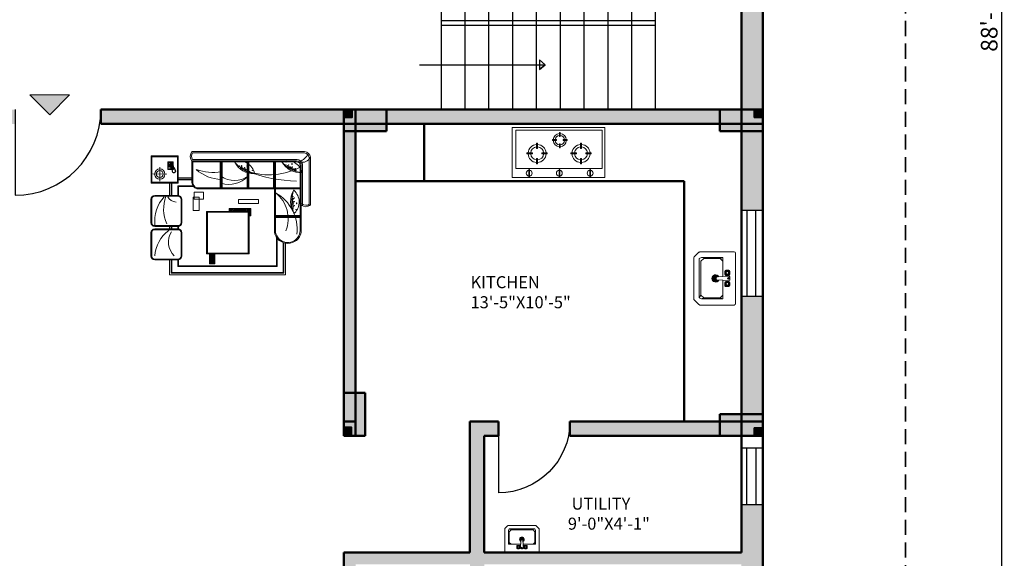
# Model space of a CAD drawing. Units: inches. Extents: x -7 to 1228, y -146 to 1091.
# Tile 42 of 88: x 815 to 1228, y 304 to 531. Entities that reach past the tile are written whole.
import ezdxf

# ---------------------------------------------------------------- set-up
doc = ezdxf.new("R2010")
doc.units = ezdxf.units.IN
doc.linetypes.add('DASHED2', pattern=[9.525, 6.35, -3.175])
for name, color, linetype, lineweight in [('A-ANNO-DIMS', 2, 'Continuous', 18), ('A-ANNO-SYMB', 30, 'Continuous', 18), ('A-AREA-IDEN', 7, 'Continuous', 18), ('A-COLS', 6, 'Continuous', 35), ('A-DOOR', 4, 'Continuous', 25), ('A-FLOR-STRS', 1, 'Continuous', 25), ('A-FURN', 8, 'Continuous', 18), ('A-GLAZ', 175, 'Continuous', 25), ('A-WALL', 7, 'Continuous', 50), ('A-WALL-PATT', 251, 'Continuous', 13), ('C-PROP', 1, 'DASHED2', 35)]:
    doc.layers.add(name, color=color, linetype=linetype, lineweight=lineweight)
doc.styles.get("Standard").update_dxf_attribs({"font": 'arial.ttf'})
doc.dimstyles.new('ISO-25', dxfattribs={"dimtxt": 7, "dimasz": 4, "dimexe": 1.25, "dimexo": 0.625, "dimtad": 1, "dimdec": 1, "dimlunit": 3, "dimtxsty": 'Standard', "dimcen": 2.5, "dimadec": 0, "dimazin": 0, "dimtfac": 1, "dimtdec": 1, "dimtmove": 1, "dimatfit": 3, "dimfxl": 1, "dimarcsym": 0})

# ---------------------------------------------------------------- blocks, each defined once
blk = doc.blocks.new('A$C72243D80')
at = {"ltscale": 1000}
for p, q in [((0, 0), (0, 384.2)), ((0, 384.2), (712, 384.2)), ((712, 384.2), (712, 0)), ((29.5, 68.9), (29.5, 363.2)), ((29.5, 363.2), (692.7, 363.2)), ((363.5, 314.5), (363.5, 345.1)), ((363.5, 345.1), (369.5, 345.1)), ((369.5, 314.5), (363.5, 314.5)), ((369.5, 345.1), (369.5, 314.5)), ((692.7, 363.2), (692.7, 68.9)), ((188.1, 264.2), (188.1, 222.1)), ((196.4, 264.2), (188.1, 264.2)), ((196.4, 222.1), (196.4, 264.2)), ((309.4, 291), (340, 291)), ((309.4, 285), (309.4, 291)), ((340, 285), (309.4, 285)), ((340, 291), (340, 285)), ((363.5, 260), (363.5, 229.4)), ((369.5, 260), (363.5, 260)), ((363.5, 229.4), (369.5, 229.4)), ((369.5, 229.4), (369.5, 260)), ((392.3, 291), (392.3, 285)), ((422.9, 291), (392.3, 291)), ((392.3, 285), (422.9, 285)), ((422.9, 285), (422.9, 291)), ((525.9, 222.1), (525.9, 264.2)), ((525.9, 264.2), (534.1, 264.2)), ((534.1, 264.2), (534.1, 222.1)), ((114.7, 189.8), (156.8, 189.8)), ((114.7, 181.6), (114.7, 189.8)), ((156.8, 181.6), (114.7, 181.6)), ((156.8, 189.8), (156.8, 181.6)), ((188.1, 222.1), (196.4, 222.1)), ((228.6, 189.8), (228.6, 181.6)), ((270.7, 189.8), (228.6, 189.8)), ((228.6, 181.6), (270.7, 181.6)), ((270.7, 181.6), (270.7, 189.8)), ((451.5, 189.8), (493.6, 189.8)), ((451.5, 181.6), (451.5, 189.8)), ((493.6, 181.6), (451.5, 181.6)), ((493.6, 189.8), (493.6, 181.6)), ((534.1, 222.1), (525.9, 222.1)), ((565.5, 189.8), (565.5, 181.6)), ((607.6, 189.8), (565.5, 189.8)), ((565.5, 181.6), (607.6, 181.6)), ((607.6, 181.6), (607.6, 189.8)), ((188.1, 147.2), (196.4, 147.2)), ((188.1, 105.1), (188.1, 147.2)), ((196.4, 105.1), (188.1, 105.1)), ((196.4, 147.2), (196.4, 105.1)), ((525.9, 147.2), (525.9, 105.1)), ((534.1, 147.2), (525.9, 147.2)), ((525.9, 105.1), (534.1, 105.1)), ((534.1, 105.1), (534.1, 147.2)), ((712, 0), (0, 0)), ((692.7, 68.9), (29.5, 68.9)), ((129.6, 61.1), (129.6, 5)), ((134.4, 61.1), (129.6, 61.1)), ((129.6, 5), (134.4, 5)), ((134.4, 5), (134.4, 61.1)), ((360.9, 5), (360.9, 61.1)), ((360.9, 61.1), (365.7, 61.1)), ((365.7, 5), (360.9, 5)), ((365.7, 61.1), (365.7, 5)), ((597, 5), (597, 61.1)), ((597, 61.1), (601.8, 61.1)), ((601.8, 5), (597, 5)), ((601.8, 61.1), (601.8, 5))]:
    blk.add_line(p, q, dxfattribs=at)
for centre, radius, start, end in [((366.2, 287.2), 50.3, 93.03445, 175.72709), ((366.1, 287.8), 36.3, 94.03738, 175.01421), ((366.2, 287.2), 50.3, 4.27291, 86.18384), ((366.1, 287.8), 36.3, 4.98579, 84.5356), ((192.7, 184.7), 69.2, 93.81616, 175.72709), ((192.9, 185.5), 49.9, 95.4644, 175.01421), ((192.7, 184.7), 69.2, 4.27291, 86.96555), ((192.9, 185.5), 49.9, 4.98579, 85.96262), ((366.2, 287.2), 50.3, 182.57829, 266.96555), ((366.1, 287.8), 36.3, 184.51534, 265.96262), ((366.1, 287.8), 36.3, 275.4644, 355.48466), ((366.2, 287.2), 50.3, 273.81616, 357.42171), ((529.5, 184.7), 69.2, 93.03445, 175.72709), ((529.4, 185.5), 49.9, 94.03738, 175.01421), ((529.5, 184.7), 69.2, 4.27291, 86.18384), ((529.4, 185.5), 49.9, 4.98579, 84.5356), ((192.7, 184.7), 69.2, 182.57829, 266.18384), ((192.9, 185.5), 49.9, 184.51534, 264.5356), ((192.9, 185.5), 49.9, 274.03738, 355.48466), ((192.7, 184.7), 69.2, 273.03445, 357.42171), ((529.5, 184.7), 69.2, 182.57829, 266.96555), ((529.4, 185.5), 49.9, 184.51534, 265.96262), ((529.5, 184.7), 69.2, 273.81616, 357.42171), ((529.4, 185.5), 49.9, 275.4644, 355.48466), ((132.3, 33.2), 22.5, 96.74526, 263.25474), ((132.3, 33.2), 22.5, 275.47893, 84.52107), ((363.1, 33.2), 22.5, 95.47893, 264.52107), ((363.1, 33.2), 22.5, 276.74526, 83.25474), ((599.2, 33.2), 22.5, 95.47893, 264.52107), ((599.2, 33.2), 22.5, 276.74526, 83.25474)]:
    blk.add_arc(centre, radius, start, end, dxfattribs=at)
blk = doc.blocks.new('A$C4CB854FF')
for p, q in [((0, 0.3675), (0, 0.0552)), ((0.4725, 0.38), (0.0125, 0.38)), ((0.485, 0.0552), (0.485, 0.3675)), ((0.1677, 0.2932), (0.1677, 0.318)), ((0.1745, 0.2919), (0.1745, 0.3194)), ((0.1773, 0.3221), (0.2048, 0.3221)), ((0.2048, 0.2891), (0.1773, 0.2891)), ((0.1787, 0.329), (0.2034, 0.329)), ((0.2034, 0.2822), (0.1787, 0.2822)), ((0.2075, 0.3194), (0.2075, 0.2919)), ((0.2144, 0.318), (0.2144, 0.2932)), ((0.2279, 0.2104), (0.2213, 0.3235)), ((0.2337, 0.329), (0.2502, 0.329)), ((0.2625, 0.3235), (0.256, 0.2104)), ((0.2694, 0.318), (0.2694, 0.2932)), ((0.2763, 0.3194), (0.2763, 0.2919)), ((0.3065, 0.3221), (0.279, 0.3221)), ((0.279, 0.2891), (0.3065, 0.2891)), ((0.3052, 0.329), (0.2804, 0.329)), ((0.2804, 0.2822), (0.3052, 0.2822)), ((0.3093, 0.2919), (0.3093, 0.3194)), ((0.3162, 0.2932), (0.3162, 0.318)), ((0.05, 0.265), (0.2247, 0.265)), ((0.06, 0.24), (0.05, 0.265)), ((0.05, 0.07), (0.05, 0.265)), ((0.085, 0.265), (0.06, 0.24)), ((0.06, 0.24), (0.06, 0.09)), ((0.2152, 0.1984), (0.2694, 0.1984)), ((0.2297, 0.2066), (0.2165, 0.2066)), ((0.2681, 0.1901), (0.2165, 0.1901)), ((0.2272, 0.2149), (0.2208, 0.2149)), ((0.2638, 0.1819), (0.2208, 0.1819)), ((0.2505, 0.2052), (0.2334, 0.2052)), ((0.2681, 0.2066), (0.2541, 0.2066)), ((0.2638, 0.2149), (0.2566, 0.2149)), ((0.2591, 0.265), (0.43, 0.265)), ((0.395, 0.265), (0.42, 0.24)), ((0.42, 0.24), (0.43, 0.265)), ((0.42, 0.24), (0.42, 0.09)), ((0.43, 0.07), (0.43, 0.265)), ((0.06, 0.09), (0.085, 0.065)), ((0.2533, 0.1736), (0.2313, 0.1736)), ((0.42, 0.09), (0.395, 0.065)), ((0.42, 0.09), (0.43, 0.07)), ((0.0037, 0.0463), (0.0463, 0.0037)), ((0.05, 0.07), (0.06, 0.05)), ((0.42, 0.05), (0.06, 0.05)), ((0.085, 0.065), (0.395, 0.065)), ((0.395, 0.065), (0.42, 0.05)), ((0.43, 0.07), (0.42, 0.05)), ((0.4387, 0.0037), (0.4813, 0.0463)), ((0.0552, 0), (0.4298, 0))]:
    blk.add_line(p, q)
for centre, radius in [((0.191, 0.3056), 0.0165), ((0.191, 0.3056), 0.0127), ((0.2419, 0.3152), 0.00688), ((0.2419, 0.3152), 0.00344), ((0.2928, 0.3056), 0.0165), ((0.2928, 0.3056), 0.0127)]:
    blk.add_circle(centre, radius)
for centre, radius, start, end in [((0.0125, 0.3675), 0.0125, 90, 180), ((0.4725, 0.3675), 0.0125, 0, 90), ((0.1787, 0.318), 0.011, 90, 180), ((0.1787, 0.2932), 0.011, 180, 270), ((0.1773, 0.3194), 0.00275, 90, 180), ((0.1773, 0.2919), 0.00275, 180, 270), ((0.2034, 0.318), 0.011, 0, 90), ((0.2034, 0.2932), 0.011, 270, 0), ((0.2048, 0.3194), 0.00275, 360, 90), ((0.2048, 0.2919), 0.00275, 270, 0), ((0.2329, 0.314), 0.015, 87.19754, 140.72744), ((0.2509, 0.314), 0.015, 39.27256, 92.80246), ((0.2804, 0.318), 0.011, 90, 180), ((0.2804, 0.2932), 0.011, 180, 270), ((0.279, 0.3194), 0.00275, 90, 180), ((0.279, 0.2919), 0.00275, 180, 270), ((0.3052, 0.318), 0.011, 0, 90), ((0.3052, 0.2932), 0.011, 270, 360), ((0.3065, 0.3194), 0.00275, 360, 90), ((0.3065, 0.2919), 0.00275, 270, 0), ((0.2423, 0.1984), 0.033, 118.68833, 62.86857), ((0.2423, 0.1984), 0.0271, 124.77581, 57.22467), ((0.2334, 0.2107), 0.0055, 183.3274, 270), ((0.2505, 0.2107), 0.0055, 270, 356.6726), ((0.0125, 0.0552), 0.0125, 180, 225), ((0.0552, 0.0125), 0.0125, 225, 270), ((0.4298, 0.0125), 0.0125, 270, 315), ((0.4725, 0.0552), 0.0125, 315, 0)]:
    blk.add_arc(centre, radius, start, end)
blk = doc.blocks.new('*D12')
at = {"layer": 'A-ANNO-DIMS', "color": 0, "lineweight": -2, "transparency": 16777216}
for p, q in [((1187.62, 1061), (1228.45, 1061)), ((1227.2, 1057), (1227.2, 4)), ((1187.62, 0), (1228.45, 0))]:
    blk.add_line(p, q, dxfattribs=at)
at = {"layer": 'A-ANNO-DIMS', "color": 0, "transparency": 16777216}
for points in [[(1226.53, 1057), (1227.86, 1057), (1227.2, 1061)], [(1226.53, 4), (1227.86, 4), (1227.2, 0)]]:
    blk.add_solid(points, dxfattribs=at)
at = {"layer": 'Defpoints', "color": 0, "transparency": 16777216}
for p in [(1187, 1061), (1187, 0), (1227.2, 0)]:
    blk.add_point(p, dxfattribs=at)
at = {"layer": 'A-ANNO-DIMS', "color": 0, "transparency": 16777216, "insert": (1223, 530.5), "char_height": 7, "attachment_point": 5, "rotation": 90}
blk.add_mtext('88\'-5"', dxfattribs=at)
blk = doc.blocks.new('A$C327A19D4')
for p, q in [((703, 3073), (3, 3073)), ((3, 3073), (3, 2373)), ((703, 2373), (703, 3073)), ((1059, 3191), (3976, 3191)), ((1078, 3155), (3976, 3155)), ((683, 3053), (23, 3053)), ((23, 3053), (23, 2393)), ((683, 2393), (683, 3053)), ((1056, 2949), (3763, 2949)), ((1056, 2403), (1056, 2949)), ((1056, 2925), (3763, 2925)), ((1076, 2985), (3780, 2985)), ((1080, 2403), (1080, 2949)), ((1791, 2223), (1791, 2949)), ((1815, 2465), (1815, 2949)), ((1815, 2223), (1815, 2872)), ((1815, 2223), (1815, 2872)), ((1815, 2465), (1815, 2872)), ((1815, 2465), (1815, 2872)), ((1839, 2223), (1839, 2949)), ((2487, 2223), (2487, 2949)), ((2511, 2223), (2511, 2949)), ((2535, 2223), (2535, 2949)), ((3169, 2223), (3169, 2949)), ((3193, 2465), (3193, 2949)), ((3193, 2223), (3193, 2872)), ((3193, 2223), (3193, 2872)), ((3193, 2465), (3193, 2872)), ((3193, 2465), (3193, 2872)), ((3221, 1195), (3221, 2949)), ((3860, 2828), (3860, 1185)), ((3884, 2828), (3884, 1095)), ((3920, 2867), (3920, 1802)), ((4090, 3043), (4090, 1800)), ((4126, 3043), (4126, 1800)), ((49, 2607), (409, 2603)), ((231, 2784), (227, 2425)), ((3, 2373), (703, 2373)), ((23, 2393), (683, 2393)), ((484, 2052), (484, 2373)), ((524, 2052), (524, 2373)), ((544, 2052), (544, 2373)), ((694, 2052), (694, 2302)), ((694, 2302), (1084, 2302)), ((703, 2512), (1056, 2512)), ((703, 2472), (1056, 2472)), ((703, 2452), (1056, 2452)), ((714, 2051), (714, 2282)), ((714, 2282), (1098, 2282)), ((1119, 2135), (1357, 2135)), ((1119, 1958), (1119, 2135)), ((3884, 2247), (1184, 2247)), ((3884, 2223), (1184, 2223)), ((1357, 2135), (1357, 1958)), ((3195, 2235), (3195, 1095)), ((1092, 2007), (1244, 2007)), ((1092, 1659), (1092, 2007)), ((1357, 1958), (1119, 1958)), ((1244, 2007), (1244, 1659)), ((2265, 1945), (2780, 1945)), ((2265, 1845), (2265, 1945)), ((2780, 1845), (2265, 1845)), ((2780, 1945), (2780, 1845)), ((1244, 1659), (1092, 1659)), ((2539, 1638), (1439, 1638)), ((1439, 1638), (1439, 538)), ((2519, 1618), (1459, 1618)), ((1459, 1618), (1459, 558)), ((2023, 1638), (2023, 1711)), ((2023, 1711), (2585, 1711)), ((2519, 558), (2519, 1618)), ((2539, 538), (2539, 1638)), ((2585, 1711), (2585, 1522)), ((3884, 1532), (3195, 1532)), ((2585, 1522), (2539, 1522)), ((3884, 1508), (3195, 1508)), ((3884, 1484), (3195, 1484)), ((484, 1185), (484, 1252)), ((524, 1185), (524, 1252)), ((544, 1185), (544, 1252)), ((694, 1185), (694, 1252)), ((714, 1184), (714, 1253)), ((3247, 967), (3247, 230)), ((3267, 940), (3267, 210)), ((3417, 832), (3417, 60)), ((3437, 825), (3437, 40)), ((3477, 816), (3477, 0)), ((1439, 538), (2539, 538)), ((1459, 558), (2519, 558)), ((1516, 538), (1651, 538)), ((1516, 285), (1516, 538)), ((1651, 538), (1651, 285)), ((484, 0), (484, 385)), ((524, 40), (524, 385)), ((544, 60), (544, 385)), ((694, 210), (694, 385)), ((714, 230), (714, 386)), ((1651, 285), (1516, 285)), ((3437, 40), (524, 40)), ((3417, 60), (544, 60)), ((3267, 210), (694, 210)), ((3247, 230), (714, 230)), ((3477, 0), (484, 0))]:
    blk.add_line(p, q)
at = {"linetype": 'ByBlock'}
for p, q in [((438, 2915), (440, 2918)), ((439, 2728), (438, 2915)), ((440, 2918), (576, 2919)), ((451, 2906), (490, 2906)), ((451, 2856), (451, 2906)), ((491, 2856), (451, 2856)), ((453, 2831), (453, 2839)), ((453, 2839), (461, 2839)), ((461, 2831), (453, 2831)), ((453, 2824), (461, 2825)), ((453, 2816), (453, 2824)), ((461, 2816), (453, 2816)), ((453, 2801), (453, 2810)), ((453, 2810), (461, 2810)), ((461, 2839), (461, 2831)), ((461, 2825), (461, 2816)), ((461, 2810), (461, 2802)), ((466, 2839), (475, 2840)), ((467, 2831), (466, 2839)), ((475, 2831), (467, 2831)), ((467, 2816), (467, 2825)), ((467, 2825), (475, 2825)), ((475, 2817), (467, 2816)), ((467, 2802), (467, 2810)), ((467, 2810), (475, 2810)), ((475, 2840), (475, 2831)), ((475, 2825), (475, 2817)), ((475, 2810), (475, 2802)), ((480, 2840), (488, 2840)), ((480, 2831), (480, 2840)), ((488, 2832), (480, 2831)), ((480, 2817), (480, 2825)), ((480, 2825), (488, 2825)), ((488, 2817), (480, 2817)), ((480, 2810), (488, 2810)), ((480, 2802), (480, 2810)), ((488, 2840), (488, 2832)), ((488, 2825), (488, 2817)), ((488, 2810), (488, 2802)), ((490, 2906), (491, 2856)), ((505, 2903), (494, 2903)), ((494, 2903), (494, 2899)), ((494, 2899), (505, 2899)), ((495, 2895), (495, 2891)), ((505, 2895), (495, 2895)), ((495, 2891), (505, 2891)), ((495, 2887), (495, 2883)), ((505, 2887), (495, 2887)), ((495, 2883), (505, 2883)), ((495, 2879), (495, 2875)), ((505, 2879), (495, 2879)), ((495, 2875), (505, 2875)), ((495, 2871), (495, 2867)), ((506, 2871), (495, 2871)), ((495, 2867), (506, 2867)), ((495, 2863), (495, 2859)), ((506, 2863), (495, 2863)), ((495, 2859), (506, 2859)), ((505, 2899), (505, 2903)), ((505, 2891), (505, 2895)), ((505, 2883), (505, 2887)), ((505, 2875), (505, 2879)), ((506, 2867), (506, 2871)), ((506, 2859), (506, 2863)), ((515, 2908), (520, 2914)), ((516, 2744), (515, 2908)), ((520, 2910), (519, 2905)), ((519, 2905), (531, 2893)), ((519, 2905), (519, 2868)), ((519, 2868), (522, 2862)), ((520, 2914), (561, 2915)), ((526, 2913), (520, 2910)), ((522, 2862), (526, 2855)), ((532, 2895), (526, 2913)), ((526, 2913), (558, 2913)), ((526, 2855), (527, 2845)), ((526, 2797), (528, 2806)), ((527, 2845), (527, 2832)), ((528, 2806), (527, 2832)), ((531, 2893), (532, 2895)), ((532, 2832), (531, 2893)), ((551, 2896), (532, 2895)), ((532, 2832), (532, 2759)), ((551, 2896), (558, 2913)), ((553, 2893), (551, 2896)), ((565, 2905), (553, 2893)), ((553, 2832), (553, 2893)), ((553, 2832), (554, 2759)), ((558, 2855), (557, 2846)), ((557, 2846), (557, 2832)), ((557, 2806), (557, 2832)), ((559, 2797), (557, 2806)), ((558, 2913), (563, 2911)), ((562, 2862), (558, 2855)), ((561, 2915), (568, 2908)), ((565, 2869), (562, 2862)), ((563, 2911), (565, 2905)), ((565, 2905), (565, 2869)), ((568, 2908), (569, 2745)), ((576, 2919), (578, 2916)), ((578, 2916), (580, 2729)), ((442, 2726), (439, 2728)), ((543, 2726), (442, 2726)), ((461, 2802), (453, 2801)), ((453, 2787), (453, 2795)), ((453, 2795), (461, 2795)), ((461, 2787), (453, 2787)), ((468, 2743), (455, 2743)), ((455, 2743), (455, 2735)), ((455, 2735), (469, 2735)), ((461, 2795), (461, 2787)), ((475, 2802), (467, 2802)), ((467, 2787), (467, 2795)), ((467, 2795), (475, 2795)), ((475, 2787), (467, 2787)), ((469, 2735), (468, 2743)), ((487, 2743), (474, 2743)), ((474, 2743), (474, 2735)), ((474, 2735), (487, 2735)), ((475, 2795), (475, 2787)), ((488, 2802), (480, 2802)), ((480, 2787), (480, 2795)), ((480, 2795), (488, 2795)), ((488, 2787), (480, 2787)), ((487, 2735), (487, 2743)), ((488, 2795), (488, 2787)), ((493, 2744), (493, 2735)), ((506, 2744), (493, 2744)), ((493, 2735), (506, 2735)), ((497, 2795), (507, 2795)), ((497, 2787), (497, 2795)), ((507, 2787), (497, 2787)), ((506, 2735), (506, 2744)), ((507, 2795), (507, 2787)), ((523, 2737), (516, 2744)), ((520, 2783), (522, 2790)), ((520, 2746), (520, 2783)), ((520, 2746), (532, 2759)), ((521, 2741), (520, 2746)), ((527, 2738), (521, 2741)), ((522, 2790), (526, 2797)), ((542, 2737), (523, 2737)), ((533, 2756), (527, 2738)), ((527, 2738), (542, 2738)), ((532, 2759), (533, 2756)), ((552, 2756), (533, 2756)), ((546, 2743), (542, 2743)), ((542, 2743), (542, 2731)), ((542, 2731), (545, 2717)), ((545, 2717), (549, 2704)), ((547, 2732), (546, 2743)), ((546, 2738), (559, 2739)), ((562, 2737), (546, 2737)), ((549, 2696), (546, 2692)), ((546, 2692), (546, 2686)), ((546, 2686), (554, 2685)), ((554, 2685), (546, 2680)), ((546, 2680), (547, 2672)), ((548, 2723), (547, 2732)), ((547, 2672), (555, 2672)), ((577, 2726), (548, 2726)), ((552, 2710), (548, 2723)), ((549, 2704), (548, 2697)), ((548, 2697), (549, 2696)), ((555, 2672), (548, 2666)), ((548, 2666), (551, 2659)), ((551, 2659), (560, 2661)), ((554, 2759), (552, 2756)), ((552, 2756), (559, 2739)), ((553, 2703), (552, 2710)), ((552, 2696), (553, 2703)), ((557, 2693), (552, 2696)), ((566, 2747), (554, 2759)), ((556, 2687), (557, 2693)), ((558, 2669), (556, 2687)), ((560, 2661), (556, 2653)), ((556, 2653), (560, 2648)), ((568, 2656), (558, 2669)), ((563, 2790), (559, 2797)), ((559, 2739), (565, 2741)), ((560, 2648), (566, 2653)), ((569, 2745), (562, 2737)), ((566, 2783), (563, 2790)), ((565, 2741), (566, 2747)), ((566, 2653), (565, 2646)), ((565, 2646), (570, 2642)), ((566, 2747), (566, 2783)), ((583, 2649), (568, 2656)), ((570, 2642), (577, 2648)), ((577, 2648), (576, 2639)), ((576, 2639), (582, 2637)), ((580, 2729), (577, 2726)), ((587, 2779), (579, 2779)), ((579, 2775), (584, 2774)), ((582, 2637), (585, 2645)), ((599, 2647), (583, 2649)), ((584, 2774), (587, 2772)), ((585, 2645), (589, 2637)), ((590, 2777), (587, 2779)), ((587, 2772), (591, 2770)), ((589, 2637), (593, 2637)), ((594, 2771), (590, 2777)), ((591, 2770), (593, 2768)), ((595, 2768), (592, 2765)), ((592, 2765), (597, 2757)), ((593, 2768), (595, 2768)), ((593, 2637), (595, 2645)), ((599, 2771), (594, 2771)), ((595, 2645), (598, 2636)), ((597, 2757), (606, 2742)), ((598, 2636), (604, 2637)), ((602, 2770), (599, 2771)), ((599, 2760), (603, 2767)), ((606, 2763), (599, 2760)), ((615, 2654), (599, 2647)), ((603, 2767), (602, 2770)), ((604, 2750), (608, 2758)), ((612, 2753), (604, 2750)), ((604, 2645), (610, 2639)), ((604, 2637), (604, 2645)), ((608, 2758), (606, 2763)), ((606, 2742), (612, 2731)), ((608, 2742), (614, 2749)), ((615, 2746), (608, 2742)), ((610, 2639), (615, 2642)), ((614, 2749), (612, 2753)), ((612, 2731), (614, 2730)), ((613, 2733), (618, 2740)), ((621, 2736), (613, 2733)), ((614, 2730), (613, 2728)), ((613, 2728), (622, 2712)), ((614, 2650), (619, 2643)), ((615, 2642), (614, 2650)), ((618, 2740), (615, 2746)), ((627, 2666), (615, 2654)), ((619, 2643), (624, 2647)), ((620, 2723), (624, 2730)), ((627, 2725), (620, 2723)), ((620, 2654), (628, 2651)), ((624, 2647), (620, 2654)), ((624, 2730), (621, 2736)), ((622, 2712), (631, 2687)), ((626, 2712), (630, 2720)), ((634, 2713), (626, 2712)), ((630, 2720), (627, 2725)), ((631, 2687), (627, 2666)), ((628, 2702), (636, 2705)), ((637, 2702), (628, 2702)), ((628, 2661), (636, 2659)), ((632, 2654), (628, 2661)), ((628, 2651), (632, 2654)), ((631, 2672), (640, 2672)), ((638, 2665), (631, 2672)), ((633, 2691), (639, 2696)), ((641, 2691), (633, 2691)), ((636, 2705), (634, 2713)), ((634, 2681), (642, 2684)), ((641, 2677), (634, 2681)), ((636, 2659), (638, 2665)), ((639, 2696), (637, 2702)), ((640, 2672), (641, 2677)), ((642, 2684), (641, 2691))]:
    blk.add_line(p, q, dxfattribs=at)
at = {"ltscale": 5}
for p, q in [((100, 2052), (700, 2052)), ((0, 1352), (0, 1952)), ((20, 1352), (20, 1952)), ((100, 2032), (700, 2032)), ((780, 1952), (780, 1352)), ((800, 1952), (800, 1352)), ((2023, 1673), (2061, 1711)), ((2027, 1638), (2100, 1711)), ((2067, 1638), (2139, 1711)), ((2106, 1638), (2179, 1711)), ((2145, 1638), (2218, 1711)), ((2184, 1638), (2257, 1711)), ((2224, 1638), (2296, 1711)), ((2263, 1638), (2336, 1711)), ((2302, 1638), (2375, 1711)), ((2341, 1638), (2414, 1711)), ((2381, 1638), (2453, 1711)), ((2420, 1638), (2493, 1711)), ((2459, 1638), (2532, 1711)), ((2498, 1638), (2571, 1711)), ((2538, 1638), (2585, 1685)), ((2539, 1601), (2585, 1646)), ((2539, 1561), (2585, 1607)), ((2539, 1522), (2585, 1568)), ((2578, 1522), (2585, 1528)), ((0, 485), (0, 1085)), ((20, 485), (20, 1085)), ((700, 1272), (100, 1272)), ((700, 1252), (100, 1252)), ((100, 1185), (700, 1185)), ((100, 1165), (700, 1165)), ((780, 1085), (780, 485)), ((800, 1085), (800, 485)), ((1516, 499), (1555, 538)), ((1516, 460), (1594, 538)), ((1516, 421), (1634, 538)), ((1516, 382), (1651, 516)), ((700, 405), (100, 405)), ((700, 385), (100, 385)), ((1516, 342), (1651, 477)), ((1516, 303), (1651, 438)), ((1537, 285), (1651, 398)), ((1576, 285), (1651, 359)), ((1616, 285), (1651, 320))]:
    blk.add_line(p, q, dxfattribs=at)
for radius in [134, 88.7]:
    blk.add_circle((229, 2605), radius)
for centre, radius, start, end in [((1218, 3068), 201, 142.4201, 216.3682), ((1218, 3068), 165, 148.4003, 210.2229), ((3657, 3353), 468, 293.6733, 332.9672), ((3943, 3007), 150, 10.9855, 79.893), ((3943, 3007), 187, 10.9855, 79.893), ((2545, 3192), 468, 214.7097, 257.8799), ((2283, 2531), 409, 13.4523, 105.9639), ((2657, 3163), 547, 207.1715, 271.8037), ((3869, 3188), 547, 208.8478, 273.48), ((3911, 3323), 657, 217.6007, 253.5739), ((3517, 2544), 409, 14.6876, 107.1992), ((3763, 2828), 157, 0, 90), ((3763, 2828), 121, 0, 90), ((3763, 2828), 96.8, 0, 90), ((3921, 3138), 226, 250.4844, 335.1673), ((1594, 3859), 1211, 249.7283, 280.5443), ((1853, 3485), 1021, 228.2765, 267.8541), ((2024, 3008), 670, 251.8392, 316.629), ((2163, 3036), 599, 234.5154, 305.4846), ((2752, 3267), 657, 227.0776, 263.0508), ((3052, 4350), 1764, 252.1519, 298.1592), ((3865, 6197), 3777, 248.9971, 268.5461), ((3951, 3106), 468, 222.7716, 265.9418), ((1243, 2401), 187, 179.2584, 251.6848), ((1243, 2401), 163, 179.2584, 251.6848), ((4159, 1898), 547, 149.1529, 213.7851), ((4124, 2008), 468, 156.691, 199.8613), ((3425, 1881), 409, 315.4337, 47.9453), ((4298, 1873), 657, 169.059, 205.0321), ((4007, 1962), 201, 232.4201, 306.3682), ((4007, 1962), 165, 232.4201, 306.3682)]:
    blk.add_arc(centre, radius, start, end)
for centre, radius, start, end in [((100, 1952), 100, 90, 180), ((700, 1952), 100, 0, 90), ((100, 1952), 80, 90, 180), ((1024, 1388), 928, 137.1341, 186.5635), ((1307, 1706), 979, 160.9364, 203.1944), ((676, 2156), 279, 209.1633, 264.4137), ((700, 1952), 80, 0, 90), ((100, 1352), 100, 180, 270), ((100, 1352), 80, 180, 270), ((700, 1352), 80, 270, 0), ((700, 1352), 100, 270, 0), ((100, 1085), 100, 90, 180), ((100, 1085), 80, 90, 180), ((968, 436), 868, 125.4807, 176.5616), ((949, 846), 497, 147.8484, 226.1244), ((700, 1085), 100, 0, 90), ((700, 1085), 80, 0, 90), ((100, 485), 100, 180, 270), ((100, 485), 80, 180, 270), ((700, 485), 100, 270, 0), ((700, 485), 80, 270, 0)]:
    blk.add_arc(centre, radius, start, end, dxfattribs=at)
at = {"ltscale": 20}
for centre, radius, start, end in [((2701, 1449), 849, 338.2682, 52.2695), ((2703, 1175), 1078, 353.1988, 61.2564), ((3540, 1161), 351, 190.8398, 349.1602), ((3540, 1156), 321, 172.9078, 5.2194)]:
    blk.add_arc(centre, radius, start, end, dxfattribs=at)
for p in [(2298, 2818), (2345, 2825), (2485, 2814), (2498, 2803), (3492, 2920), (3495, 2842), (3535, 2825), (3560, 2838), (3641, 2868), (3657, 2862), (2329, 2780), (2344, 2802), (2356, 2781), (2375, 2736), (2410, 2757), (2421, 2774), (2421, 2720), (2444, 2738), (2445, 2691), (2459, 2715), (2481, 2700), (2514, 2718), (2515, 2690), (2551, 2664), (2620, 2701), (3561, 2800), (3571, 2765), (3585, 2789), (3609, 2758), (3612, 2788), (3646, 2728), (3647, 2768), (3655, 2787), (3694, 2735), (3707, 2710), (3719, 2734), (3738, 2747), (3756, 2703), (3646, 1828), (3648, 1911), (3658, 1864), (3660, 1974), (3673, 1803), (3674, 1829), (3676, 1951), (3677, 2020), (3684, 1893), (3686, 1853), (3687, 1973), (3705, 1892), (3706, 1784), (3707, 1984), (3770, 1842), (3772, 1859), (3680, 1724), (3683, 1768), (3748, 1685)]:
    blk.add_point(p)
blk = doc.blocks.new('WIN-36')
for p, q in [((0, 36), (0, 0)), ((9, 36), (0, 36)), ((2.34, 36), (2.34, 0)), ((6.14, 0), (6.14, 36)), ((9, 0), (9, 36)), ((0, 0), (9, 0)), ((2.34, 0), (6.14, 0))]:
    blk.add_line(p, q)
blk = doc.blocks.new('WIN-24')
for p, q in [((0, 0), (0, 24)), ((0, 24), (9, 24)), ((2.34, 0), (2.34, 24)), ((2.34, 24), (6.14, 24)), ((6.14, 24), (6.14, 0)), ((9, 24), (9, 0)), ((9, 0), (0, 0))]:
    blk.add_line(p, q)
blk = doc.blocks.new('DOOR-750')
blk.add_line((30, 30), (30, 0))
blk.add_arc((30, 30), 30, 180, 270)
blk = doc.blocks.new('DOOR-900')
blk.add_line((36, 0), (36, 36))
blk.add_arc((36, 0), 36, 90, 180)

msp = doc.modelspace()

# ---------------------------------------------------------------- hatches: boundary and pattern name
at = {"layer": 'A-ANNO-SYMB'}
h = msp.add_hatch(color=256, dxfattribs=at)
h.dxf.hatch_style = 1
h.paths.add_polyline_path([(819.19, 499.14), (827.53, 490.81), (835.87, 499.14)])
at = {"layer": 'A-COLS'}
h = msp.add_hatch(color=256, dxfattribs=at)
h.dxf.hatch_style = 1
h.paths.add_polyline_path([(954.55, 493), (954.55, 489.71), (951, 489.71), (951, 484), (969, 484), (969, 493)])
h = msp.add_hatch(color=256, dxfattribs=at)
h.dxf.hatch_style = 1
h.paths.add_polyline_path([(954.55, 493), (951, 493), (951, 489.71), (954.55, 489.71)])
h = msp.add_hatch(color=256, dxfattribs=at)
h.dxf.hatch_style = 1
h.paths.add_polyline_path([(1109, 493), (1109, 484), (1127, 484), (1127, 489.71), (1123.45, 489.71), (1123.45, 493)])
h = msp.add_hatch(color=256, dxfattribs=at)
h.dxf.hatch_style = 1
h.paths.add_polyline_path([(1123.45, 489.71), (1127, 489.71), (1127, 493), (1123.45, 493)])
h = msp.add_hatch(color=256, dxfattribs=at)
h.dxf.hatch_style = 1
h.paths.add_polyline_path([(951, 359.55), (954.29, 359.55), (954.29, 356), (960, 356), (960, 374), (951, 374)])
h = msp.add_hatch(color=256, dxfattribs=at)
h.dxf.hatch_style = 1
h.paths.add_polyline_path([(1123.45, 356), (1123.45, 359.29), (1127, 359.29), (1127, 365), (1109, 365), (1109, 356)])
h = msp.add_hatch(color=256, dxfattribs=at)
h.dxf.hatch_style = 1
h.paths.add_polyline_path([(951, 359.55), (951, 356), (954.29, 356), (954.29, 359.55)])
h = msp.add_hatch(color=256, dxfattribs=at)
h.dxf.hatch_style = 1
h.paths.add_polyline_path([(1123.45, 356), (1127, 356), (1127, 359.29), (1123.45, 359.29)])
at = {"layer": 'A-WALL-PATT'}
h = msp.add_hatch(color=256, dxfattribs=at)
h.dxf.hatch_style = 1
h.paths.add_polyline_path([(69, 568), (60, 568), (60, 493), (63.29, 493), (69, 493)])
h.paths.add_polyline_path([(69, 662.41), (60, 662.41), (60, 586), (69, 586)], flags=17)
h.paths.add_polyline_path([(69, 723), (184, 723), (184, 734), (179, 734), (179, 728), (69, 728), (69, 741.62), (60, 741.62), (60, 698.41), (69, 698.41)], flags=17)
h.paths.add_polyline_path([(69, 782), (231, 782), (231, 728), (231, 723), (231, 586), (236, 586), (236, 787), (69, 787), (69, 800.13), (60, 800.13), (60, 765.62), (69, 765.62)])
h.paths.add_polyline_path([(184, 842), (189, 842), (189, 848), (173, 848), (173, 842), (179, 842), (179, 787), (184, 787)])
h.paths.add_polyline_path([(118.22, 69), (69, 69), (69, 60), (118.22, 60)])
h.paths.add_polyline_path([(227, 69), (154.22, 69), (154.22, 60), (227, 60)])
h.paths.add_polyline_path([(236, 60), (232.71, 60), (227, 60), (227, 36), (236, 36)])
h.paths.add_polyline_path([(389, 60), (380, 60), (380, 36), (389, 36)])
h.paths.add_polyline_path([(384, 181), (380, 181), (380, 115), (380, 78), (384, 78)])
h.paths.add_polyline_path([(380, 115), (334.55, 115), (334.55, 109), (380, 109)])
h.paths.add_polyline_path([(274.55, 115), (236, 115), (236, 201), (232.71, 201), (231, 201), (231, 78), (236, 78), (236, 109), (274.55, 109)])
h.paths.add_polyline_path([(69, 123), (60, 123), (60, 78), (69, 78)])
h.paths.add_polyline_path([(69, 201), (60, 201), (60, 159), (69, 159)])
h.paths.add_polyline_path([(143, 219), (69, 219), (69, 213), (143, 213)], flags=17)
h.paths.add_polyline_path([(189, 219), (184, 219), (184, 274), (231, 274), (231, 219), (236, 219), (236, 279), (184, 279), (184, 297), (179, 297), (179, 279), (69, 279), (69, 290.91), (60, 290.91), (60, 262.18), (69, 262.18), (69, 274), (179, 274), (179, 219), (173, 219), (173, 213), (189, 213)])
h.paths.add_polyline_path([(69, 238.18), (60, 238.18), (60, 219), (69, 219)], flags=17)
h.paths.add_polyline_path([(69, 333), (60, 333), (60, 314.91), (69, 314.91), (69, 316.96)])
h.paths.add_polyline_path([(190, 338), (184, 338), (69, 338), (69, 333), (179, 333), (179, 327), (184, 327), (184, 333.02), (190, 333.05)])
h.paths.add_polyline_path([(69, 386.81), (60, 386.81), (60, 351), (69, 351)])
h.paths.add_polyline_path([(69, 475), (60, 475), (60, 422.81), (69, 422.81)])
h.paths.add_polyline_path([(236, 475), (231, 475), (231, 351.24), (236, 351.24)])
h.paths.add_polyline_path([(384, 475), (380, 475), (380, 362), (384, 362)])
h.paths.add_polyline_path([(547, 307), (439, 307), (439, 356), (445, 356), (445, 362), (433, 362), (433, 307), (380, 307), (380, 244), (380, 241), (384, 241), (384, 301), (433, 301), (433, 277), (439, 277), (439, 301), (547, 301)])
h.paths.add_polyline_path([(547, 241), (439, 241), (439, 247), (433, 247), (433, 235), (547, 235)])
h.paths.add_polyline_path([(450, 69), (440.29, 69), (424.89, 69), (389, 69), (389, 60), (450, 60)])
h.paths.add_polyline_path([(547, 69), (486, 69), (486, 60), (547, 60)])
h.paths.add_polyline_path([(556, 148.27), (547, 148.27), (547, 78), (556, 78)])
h.paths.add_polyline_path([(556, 223), (547, 223), (547, 195), (547, 184.27), (556, 184.27)])
h.paths.add_polyline_path([(556, 311.19), (547, 311.19), (547, 273.08), (556, 273.08)])
h.paths.add_polyline_path([(556, 344), (552.71, 344), (547, 344), (547, 335.19), (556, 335.19)])
h.paths.add_polyline_path([(556, 249.08), (547, 249.08), (547, 241), (556, 241)])
h.paths.add_polyline_path([(547, 362), (475, 362), (475, 356), (547, 356)], flags=0)
h.paths.add_polyline_path([(556, 399.62), (547, 399.62), (547, 362), (556, 362)])
h.paths.add_polyline_path([(556, 475), (547, 475), (547, 435.62), (556, 435.62)])
h.paths.add_polyline_path([(547, 493), (389, 493), (389, 487), (547, 487)])
h.paths.add_polyline_path([(380, 493), (278, 493), (278, 487), (380, 487)])
h.paths.add_polyline_path([(227, 493), (69, 493), (69, 487), (227, 487)])
h.paths.add_polyline_path([(643, 122.44), (634, 122.44), (634, 78), (643, 78)])
h.paths.add_polyline_path([(702.5, 69), (692.79, 69), (677.39, 69), (643, 69), (643, 60), (702.5, 60)])
h.paths.add_polyline_path([(798, 69), (738.5, 69), (738.5, 60), (798, 60)])
h.paths.add_polyline_path([(807, 60), (803.71, 60), (798, 60), (798, 36), (807, 36)])
h.paths.add_polyline_path([(807, 109), (846.75, 109), (846.75, 115), (807, 115), (807, 159), (802, 159), (802, 78), (807, 78)])
h.paths.add_polyline_path([(807, 201), (802, 201), (802, 195), (807, 195)])
h.paths.add_polyline_path([(643, 201), (634, 201), (634, 158.44), (643, 158.44)])
h.paths.add_polyline_path([(756, 225), (751, 225), (751, 219), (643, 219), (643, 213), (756, 213)])
h.paths.add_polyline_path([(643, 240.85), (634, 240.85), (634, 219), (643, 219)])
h.paths.add_polyline_path([(643, 274), (643, 288.63), (634, 288.63), (634, 264.85), (643, 264.85)])
h.paths.add_polyline_path([(802, 279), (756, 279), (756, 297), (751, 297), (751, 279), (643, 279), (643, 274), (751, 274), (751, 255), (756, 255), (756, 274), (802, 274)])
h.paths.add_polyline_path([(807, 333), (803.71, 333), (802, 333), (802, 279), (802, 274), (802, 219), (807, 219)])
h.paths.add_polyline_path([(956, 182), (951, 182), (951, 115), (906.75, 115), (906.75, 109), (951, 109), (951, 78), (956, 78)])
h.paths.add_polyline_path([(960, 60), (951, 60), (951, 36), (960, 36)])
h.paths.add_polyline_path([(1021, 69), (1005.78, 69), (960, 69), (960, 60), (1021, 60)])
h.paths.add_polyline_path([(956, 224), (951, 224), (951, 218), (956, 218)])
h.paths.add_polyline_path([(956, 302), (1004, 302), (1004, 278), (1010, 278), (1010, 302), (1118, 302), (1118, 290.81), (1127, 290.81), (1127, 326.97), (1118, 326.97), (1118, 320.97), (1118, 307), (1010, 307), (1010, 356), (1016, 356), (1016, 362), (1004, 362), (1004, 307), (951, 307), (951, 244), (951, 242), (954.29, 242), (956, 242)])
h.paths.add_polyline_path([(643, 333), (634, 333), (634, 312.63), (643, 312.63), (643, 316.96)])
h.paths.add_polyline_path([(756, 338), (643, 338), (643, 333), (751, 333), (751, 327), (756, 327)])
h.paths.add_polyline_path([(643, 388), (634, 388), (634, 351), (643, 351)])
h.paths.add_polyline_path([(807, 357), (802, 357), (802, 351), (807, 351)])
h.paths.add_polyline_path([(807, 475), (802, 475), (802, 393), (807, 393)])
h.paths.add_polyline_path([(643, 475), (634, 475), (634, 424), (643, 424)])
h.paths.add_polyline_path([(798, 493), (643, 493), (643, 487), (798, 487)])
h.paths.add_polyline_path([(634, 493), (556, 493), (556, 487), (634, 487)])
h.paths.add_polyline_path([(813, 493), (807, 493), (807, 487), (813, 487)])
h.paths.add_polyline_path([(951, 493), (849, 493), (849, 487), (951, 487)])
h.paths.add_polyline_path([(956, 484), (951, 484), (951, 374), (956, 374)])
h.paths.add_polyline_path([(1109, 493), (969, 493), (969, 487), (1109, 487)])
h.paths.add_polyline_path([(1127, 484), (1118, 484), (1118, 450.64), (1127, 450.64)])
h.paths.add_polyline_path([(1127, 414.64), (1118, 414.64), (1118, 365), (1127, 365)])
h.paths.add_polyline_path([(1109, 362), (1046, 362), (1046, 356), (1109, 356)], flags=17)
h.paths.add_polyline_path([(1127, 356), (1123.45, 356), (1118, 356), (1118, 350.97), (1127, 350.97)], flags=0)
h.paths.add_polyline_path([(1127, 266.81), (1118, 266.81), (1118, 262.36), (1118, 242), (1127, 242)], flags=17)
h.paths.add_polyline_path([(1118, 242), (1010, 242), (1010, 248), (1004, 248), (1004, 237), (1118, 237)])
h.paths.add_polyline_path([(1127, 224), (1118, 224), (1118, 170), (1127, 170)])
h.paths.add_polyline_path([(1127, 134), (1118, 134), (1118, 78), (1127, 78)])
h.paths.add_polyline_path([(1118, 69), (1057, 69), (1057, 60), (1118, 60)])
h.paths.add_polyline_path([(227, 571.55), (227, 574), (69, 574), (69, 568), (227, 568)])
h.paths.add_polyline_path([(380, 571.55), (380, 574), (278, 574), (278, 568), (380, 568)])
h.paths.add_polyline_path([(242, 574), (236, 574), (236, 568), (242, 568)])
h.paths.add_polyline_path([(547, 571.55), (547, 574), (389, 574), (389, 568), (547, 568)])
h.paths.add_polyline_path([(384, 733), (380, 733), (380, 586), (384, 586)])
h.paths.add_polyline_path([(556, 646), (634, 646), (634, 655), (547, 655), (547, 586), (556, 586)])
h.paths.add_polyline_path([(634, 574), (556, 574), (556, 568), (634, 568)])
h.paths.add_polyline_path([(643, 655), (634, 655), (634, 586), (643, 586)])
h.paths.add_polyline_path([(798, 574), (643, 574), (643, 568), (798, 568)])
h.paths.add_polyline_path([(643, 663.85), (634, 663.85), (634, 655), (643, 655)])
h.paths.add_polyline_path([(556, 676.97), (547, 676.97), (547, 655), (556, 655)])
h.paths.add_polyline_path([(556, 733), (547, 733), (547, 712.97), (556, 712.97)])
h.paths.add_polyline_path([(643, 710), (634, 710), (634, 699.85), (643, 699.85)])
h.paths.add_polyline_path([(807, 668), (802, 668), (802, 586), (807, 586)])
h.paths.add_polyline_path([(951, 574), (849, 574), (849, 568), (951, 568)])
h.paths.add_polyline_path([(956, 691), (951, 691), (951, 577), (956, 577)])
h.paths.add_polyline_path([(1109, 574), (969, 574), (969, 568), (1109, 568)])
h.paths.add_polyline_path([(1127, 643.4), (1118, 643.4), (1118, 577), (1127, 577)])
h.paths.add_polyline_path([(1127, 568), (1123.45, 568), (1118, 568), (1118, 493), (1127, 493)])
h.paths.add_polyline_path([(1127, 733), (1118, 733), (1118, 679.4), (1127, 679.4)])
h.paths.add_polyline_path([(1127, 777.35), (1118, 777.35), (1118, 770.04), (1118, 751), (1127, 751)], flags=17)
h.paths.add_polyline_path([(1118, 751), (1010, 751), (1010, 757), (1004, 757), (1004, 745), (1118, 745)])
h.paths.add_polyline_path([(956, 811), (1004, 811), (1004, 787), (1010, 787), (1010, 811), (1017.87, 811), (1017.87, 811.63, -0.414214), (1018.25, 812), (1031.98, 812, -0.414214), (1032.35, 811.63), (1032.35, 811), (1118, 811), (1118, 801.35), (1127, 801.35), (1127, 834.69), (1118, 834.69), (1118, 830.24), (1118, 817), (1010, 817), (1010, 866), (1016, 866), (1016, 872), (1004, 872), (1004, 817), (956, 817), (956, 866), (951, 866), (951, 751), (954.29, 751), (956, 751)])
h.paths.add_polyline_path([(1118, 872), (1046, 872), (1046, 866), (1118, 866)], flags=17)
h.paths.add_polyline_path([(1127, 924.71), (1118, 924.71), (1118, 884), (1127, 884)])
h.paths.add_polyline_path([(1127, 866), (1123.71, 866), (1118, 866), (1118, 858.69), (1127, 858.69)], flags=17)
h.paths.add_polyline_path([(956, 983), (951, 983), (951, 952), (807, 952), (807, 983), (802, 983), (802, 902), (807, 902), (807, 946), (951, 946), (951, 884), (956, 884)])
h.paths.add_polyline_path([(807, 842), (802, 842), (802, 787), (756, 787), (756, 806), (751, 806), (751, 787), (643, 787), (643, 782), (751, 782), (751, 764), (756, 764), (756, 782), (802, 782), (802, 728), (807, 728)])
h.paths.add_polyline_path([(756, 848), (643, 848), (643, 842), (751, 842), (751, 836), (756, 836)])
h.paths.add_polyline_path([(756, 734), (751, 734), (751, 728), (643, 728), (643, 723), (756, 723)])
h.paths.add_polyline_path([(643, 749.79), (634, 749.79), (634, 728), (637.29, 728), (643, 728)])
h.paths.add_polyline_path([(643, 805.41), (634, 805.41), (634, 773.79), (643, 773.79)])
h.paths.add_polyline_path([(643, 896.66), (634, 896.66), (634, 860), (637.29, 860), (643, 860)])
h.paths.add_polyline_path([(643, 842), (634, 842), (634, 829.41), (643, 829.41)])
h.paths.add_polyline_path([(643, 983), (634, 983), (634, 932.66), (643, 932.66)])
h.paths.add_polyline_path([(1127, 983), (1118, 983), (1118, 960.71), (1127, 960.71)])
h.paths.add_polyline_path([(1118, 1001), (1077.53, 1001), (1077.53, 992), (1118, 992)])
h.paths.add_polyline_path([(1041.53, 1001), (960, 1001), (960, 992), (1041.53, 992)])
h.paths.add_polyline_path([(960, 1025), (951, 1025), (951, 1001), (954.29, 1001), (960, 1001)])
h.paths.add_polyline_path([(807, 1025), (798, 1025), (798, 1001), (807, 1001)])
h.paths.add_polyline_path([(798, 1001), (738.5, 1001), (738.5, 992), (798, 992)])
h.paths.add_polyline_path([(702.5, 1001), (643, 1001), (643, 992), (702.5, 992)])
h.paths.add_polyline_path([(547, 1001), (499.11, 1001), (499.11, 992), (547, 992)])
h.paths.add_polyline_path([(463.11, 1001), (389, 1001), (389, 992), (463.11, 992)])
h.paths.add_polyline_path([(389, 1025), (380, 1025), (380, 1022), (380, 1001), (383.29, 1001), (389, 1001)])
h.paths.add_polyline_path([(236, 1025), (227, 1025), (227, 1001), (236, 1001)])
h.paths.add_polyline_path([(236, 983), (231, 983), (231, 860), (236, 860)])
h.paths.add_polyline_path([(274.55, 952), (236, 952), (236, 946), (274.55, 946)])
h.paths.add_polyline_path([(380, 952), (334.55, 952), (334.55, 946), (380, 946)])
h.paths.add_polyline_path([(384, 983), (380, 983), (380, 884), (383.29, 884), (384, 884)])
h.paths.add_polyline_path([(227, 1001), (155.01, 1001), (155.01, 992), (162.87, 992), (227, 992)])
h.paths.add_polyline_path([(119.01, 1001), (69, 1001), (69, 992), (119.01, 992)])
h.paths.add_polyline_path([(69, 983), (60, 983), (60, 922.99), (69, 922.99)])
h.paths.add_polyline_path([(69, 886.99), (60, 886.99), (60, 860), (63.29, 860), (69, 860)])
h.paths.add_polyline_path([(143, 848), (69, 848), (69, 842), (143, 842)])

# ---------------------------------------------------------------- linework, layer by layer
at = {"layer": 'A-ANNO-SYMB'}
for p, q in [((827.53, 490.81), (819.19, 499.14)), ((819.19, 499.14), (835.87, 499.14)), ((827.53, 490.81), (835.87, 499.14))]:
    msp.add_line(p, q, dxfattribs=at)
at = {"layer": 'A-COLS'}
for points in [[(951, 493), (951, 489.71), (954.55, 489.71), (954.55, 493)], [(1127, 493), (1127, 489.71), (1123.45, 489.71), (1123.45, 493)], [(951, 356), (954.29, 356), (954.29, 359.55), (951, 359.55)], [(1127, 356), (1127, 359.29), (1123.45, 359.29), (1123.45, 356)]]:
    msp.add_lwpolyline(points, close=True, dxfattribs=at)
at = {"layer": 'A-FLOR-STRS'}
for p, q in [((992, 493), (992, 568)), ((1002, 493), (1002, 568)), ((1012, 493), (1012, 568)), ((1022, 493), (1022, 568)), ((1032, 493), (1032, 568)), ((1042, 493), (1042, 568)), ((1052, 493), (1052, 568)), ((1062, 493), (1062, 568)), ((1072, 493), (1072, 568)), ((1082, 493), (1082, 568)), ((992, 530.5), (1082, 530.5)), ((992, 528.5), (1082, 528.5)), ((1033.23, 513.94), (1035.65, 511.87)), ((1033.23, 513.94), (1033.23, 509.8)), ((982.86, 511.87), (1035.65, 511.87)), ((1035.65, 511.87), (1033.23, 509.8)), ((1033.23, 509.8), (1035.65, 511.87))]:
    msp.add_line(p, q, dxfattribs=at)
at = {"layer": 'A-WALL'}
for p, q in [((1127, 60), (1127, 1001)), ((1118, 307), (1118, 811)), ((1127, 493), (849, 493)), ((849, 493), (849, 487)), ((951, 493), (951, 484)), ((969, 493), (951, 493)), ((951, 493), (951, 356)), ((951, 356), (951, 493)), ((956, 493), (956, 356)), ((956, 356), (956, 493)), ((969, 484), (969, 493)), ((1109, 484), (1109, 493)), ((1109, 493), (1127, 493)), ((1127, 493), (1127, 484)), ((1127, 487), (849, 487)), ((951, 484), (969, 484)), ((984.77, 463), (984.77, 487)), ((1127, 484), (1109, 484)), ((1094, 463), (956, 463)), ((1094, 362), (1094, 463)), ((960, 374), (951, 374)), ((951, 374), (951, 356)), ((960, 356), (960, 374)), ((960, 374), (960, 368)), ((1127, 365), (1109, 365)), ((1109, 365), (1109, 356)), ((1127, 356), (1127, 365)), ((956, 362), (951, 362)), ((1004, 307), (1004, 362)), ((1016, 362), (1004, 362)), ((1016, 356), (1016, 362)), ((1127, 362), (1046, 362)), ((1046, 356), (1046, 362)), ((956, 356), (951, 356)), ((951, 356), (960, 356)), ((956, 356), (951, 356)), ((1010, 307), (1010, 356)), ((1016, 356), (1010, 356)), ((1127, 356), (1046, 356)), ((1109, 356), (1127, 356)), ((951, 244), (951, 307)), ((951, 307), (951, 218)), ((1004, 307), (951, 307)), ((1118, 307), (1010, 307))]:
    msp.add_line(p, q, dxfattribs=at)
at = {"layer": 'C-PROP'}
msp.add_line((1187, 0), (1187, 1061), dxfattribs=at)

# ---------------------------------------------------------------- block references
at = {"layer": 'A-DOOR', "rotation": 180}
msp.add_blockref('DOOR-900', (849, 493), dxfattribs=at)
at = {"layer": 'A-DOOR', "extrusion": (0, 0, -1), "zscale": -1}
msp.add_blockref('DOOR-750', (-1046, 332), dxfattribs=at)
at = {"layer": 'A-FURN'}
for name, p, xscale, yscale, zscale in [('A$C72243D80', (1021.67, 464.44), 0.0547573419986423, 0.0547573419986423, 0.0547573419986423), ('A$C327A19D4', (870.02, 423.62), 0.016235792481004, 0.016235792481004, 0.016235792481004)]:
    msp.add_blockref(name, p, dxfattribs=dict(at, xscale=xscale, yscale=yscale, zscale=zscale))
for p, xscale, yscale, zscale, rotation in [((1098.05, 433.22), 45.99182974636398, 45.99182974636398, 45.99182974636398, 270), ((1033.08, 318.34), 29.84864686937646, 29.84864686937646, 29.84864686937646, 180)]:
    msp.add_blockref('A$C4CB854FF', p, dxfattribs=dict(at, xscale=xscale, yscale=yscale, zscale=zscale, rotation=rotation))
at = {"layer": 'A-GLAZ'}
for name, p in [('WIN-36', (1118, 414.64)), ('WIN-24', (1118, 326.97))]:
    msp.add_blockref(name, p, dxfattribs=at)

# ---------------------------------------------------------------- texts
at = {"layer": 'A-AREA-IDEN', "char_height": 5.0568, "attachment_point": 1}
for s, insert in [(' KITCHEN\\P 13\'-5"X10\'-5"', (1002.71, 423.03)), (' UTILITY\\P9\'-0"X4\'-1"', (1045.14, 330.01))]:
    msp.add_mtext_dynamic_manual_height_columns(s, width=137.2821, gutter_width=25.28, heights=[0], dxfattribs=dict(at, insert=insert))

# ---------------------------------------------------------------- dimensions: what is measured, and where the dimension line sits
at = {"layer": 'A-ANNO-DIMS'}
dim = msp.add_linear_dim(base=(1227.2, 0), p1=(1187, 1061), p2=(1187, 0), angle=90, dimstyle='ISO-25', override={"dimclrd": 0, "dimclre": 0, "dimclrt": 0}, dxfattribs=at)
dim.commit()
dim.dimension.update_dxf_attribs({"geometry": '*D12', "text_midpoint": (1223, 530.5)})

doc.saveas('drawing.dxf')
